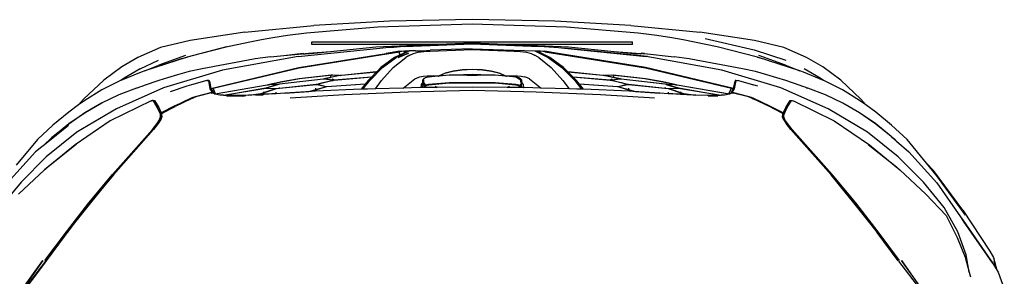
# Model space of a CAD drawing. Units: inches. Extents: x 1319 to 2030, y 219 to 1069.
# Tile 17 of 28: x 1433 to 1496, y 515 to 531. Entities that reach past the tile are written whole.
import ezdxf

# ---------------------------------------------------------------- set-up
doc = ezdxf.new("R2010")
doc.units = ezdxf.units.IN
doc.header["$MEASUREMENT"] = 0
doc.layers.get('0').update_dxf_attribs({"color": 12})
doc.layers.add('C-PRKG-VEHC', color=8, linetype='Continuous', lineweight=13)
doc.layers.add('Edges', color=250, linetype='Continuous')

# ---------------------------------------------------------------- blocks, each defined once
blk = doc.blocks.new('Nissan Qashqai pl')
at = {"layer": 'Edges'}
for p, q in [((7.6953, 12.7753), (7.7223, 12.7851)), ((7.5946, 12.718), (7.6608, 12.7617)), ((7.6113, 12.7186), (7.6759, 12.7633)), ((7.6799, 12.7658), (7.6125, 12.719)), ((7.6608, 12.7617), (7.6712, 12.7675)), ((7.6712, 12.7675), (7.6721, 12.7679)), ((7.6926, 12.7737), (7.6721, 12.7679)), ((7.6759, 12.7633), (7.6793, 12.7657)), ((7.6911, 12.7728), (7.6774, 12.7688)), ((7.6793, 12.7657), (7.6802, 12.766)), ((7.6799, 12.7658), (7.6802, 12.766)), ((7.6802, 12.766), (7.6809, 12.7664)), ((7.6809, 12.7664), (7.6911, 12.7728)), ((7.6911, 12.7728), (7.6926, 12.7737)), ((7.6926, 12.7737), (7.6953, 12.7753)), ((7.6949, 12.7283), (7.701, 12.73)), ((7.701, 12.73), (7.7024, 12.7301)), ((7.5946, 12.718), (7.5304, 12.6704)), ((7.6024, 12.7221), (7.5387, 12.6759)), ((7.5501, 12.6757), (7.6051, 12.7139)), ((7.6051, 12.7139), (7.6113, 12.7186)), ((7.6051, 12.7139), (7.6111, 12.7181)), ((7.6118, 12.7186), (7.6111, 12.7181)), ((7.6125, 12.719), (7.6118, 12.7186)), ((7.667, 12.723), (7.6295, 12.7097)), ((7.6386, 12.7089), (7.6708, 12.7217)), ((7.6949, 12.7283), (7.667, 12.723)), ((7.6708, 12.7217), (7.6949, 12.7283)), ((7.6295, 12.7097), (7.59, 12.6877)), ((7.6032, 12.6908), (7.6386, 12.7089)), ((7.59, 12.6877), (7.5492, 12.654)), ((7.5687, 12.6579), (7.6032, 12.6908)), ((7.5501, 12.6757), (7.5001, 12.6302)), ((7.5387, 12.6759), (7.5184, 12.6591)), ((7.5184, 12.6591), (7.5304, 12.6704)), ((7.5184, 12.6591), (7.4801, 12.6274)), ((7.5289, 12.6158), (7.5687, 12.6579)), ((7.5492, 12.654), (7.531, 12.6359)), ((7.7261, 12.6543), (7.6762, 12.6186)), ((7.6762, 12.6186), (7.7233, 12.6514)), ((7.531, 12.6359), (7.5081, 12.6131)), ((7.531, 12.6359), (7.5301, 12.6353)), ((7.6771, 12.6135), (7.7215, 12.6473)), ((7.4801, 12.6274), (7.4565, 12.6023)), ((7.4827, 12.6103), (7.5001, 12.6302)), ((7.4565, 12.6023), (7.4354, 12.5766)), ((7.4542, 12.5765), (7.4744, 12.6015)), ((7.475, 12.6016), (7.4549, 12.5767)), ((7.5081, 12.6131), (7.4679, 12.5634)), ((7.4744, 12.6015), (7.4804, 12.6079)), ((7.4762, 12.6028), (7.475, 12.6016)), ((7.4752, 12.6016), (7.4762, 12.6028)), ((7.4762, 12.6028), (7.478, 12.6049)), ((7.4804, 12.6079), (7.478, 12.6049)), ((7.478, 12.6049), (7.479, 12.6061)), ((7.479, 12.6061), (7.4815, 12.6089)), ((7.479, 12.6061), (7.4801, 12.6074)), ((7.4801, 12.6074), (7.4804, 12.6079)), ((7.4804, 12.6079), (7.4807, 12.6082)), ((7.4804, 12.6079), (7.4804, 12.6079)), ((7.4807, 12.6082), (7.4821, 12.6097)), ((7.4815, 12.6089), (7.4821, 12.6097)), ((7.4821, 12.6097), (7.4827, 12.6103)), ((7.4882, 12.5645), (7.5243, 12.6101)), ((7.4884, 12.5664), (7.5289, 12.6158)), ((7.5243, 12.6101), (7.5286, 12.6146)), ((7.676, 12.6152), (7.6296, 12.5803)), ((7.6769, 12.6129), (7.6306, 12.5791)), ((7.4354, 12.5766), (7.4239, 12.5604)), ((7.4363, 12.5502), (7.4542, 12.5765)), ((7.4549, 12.5767), (7.4369, 12.5504)), ((7.6296, 12.5803), (7.5827, 12.5441)), ((7.618, 12.5691), (7.5829, 12.5411)), ((7.618, 12.5691), (7.584, 12.5429)), ((7.6301, 12.5787), (7.618, 12.5691)), ((7.6306, 12.5791), (7.6301, 12.5787)), ((7.4239, 12.5604), (7.4147, 12.5524)), ((7.4239, 12.5604), (7.4166, 12.5503)), ((7.4679, 12.5634), (7.4302, 12.4993)), ((7.4498, 12.5093), (7.4884, 12.5664)), ((7.4147, 12.5524), (7.3837, 12.5197)), ((7.4166, 12.5503), (7.3997, 12.5227)), ((7.4205, 12.5229), (7.4363, 12.5502)), ((7.4369, 12.5504), (7.4211, 12.5232)), ((7.5827, 12.5441), (7.5369, 12.5057)), ((7.584, 12.5429), (7.5568, 12.5201)), ((7.5829, 12.5411), (7.5568, 12.5201)), ((7.3997, 12.5227), (7.3845, 12.4925)), ((7.4071, 12.4948), (7.4205, 12.5229)), ((7.4211, 12.5232), (7.4078, 12.4951)), ((7.3837, 12.5197), (7.3624, 12.4907)), ((7.4172, 12.4431), (7.4498, 12.5093)), ((7.5369, 12.5057), (7.4635, 12.4408)), ((7.5568, 12.5201), (7.5371, 12.5042)), ((7.3624, 12.4907), (7.347, 12.4644)), ((7.3843, 12.492), (7.3707, 12.4592)), ((7.3843, 12.492), (7.3805, 12.4866)), ((7.3845, 12.4925), (7.3843, 12.492)), ((7.3962, 12.466), (7.4071, 12.4948)), ((7.4302, 12.4993), (7.3963, 12.4227)), ((7.4078, 12.4951), (7.3969, 12.4665)), ((7.4638, 12.439), (7.5371, 12.5042)), ((7.3805, 12.4866), (7.3655, 12.4604)), ((7.347, 12.4644), (7.3309, 12.4276)), ((7.3707, 12.4592), (7.3688, 12.4532)), ((7.3938, 12.4583), (7.3925, 12.4542)), ((7.3951, 12.462), (7.3938, 12.4583)), ((7.3965, 12.4655), (7.3951, 12.462)), ((7.3965, 12.4655), (7.3962, 12.466)), ((7.3969, 12.4665), (7.3965, 12.4655)), ((7.3968, 12.4649), (7.3967, 12.4651)), ((7.3688, 12.4532), (7.3467, 12.3846)), ((7.3596, 12.4302), (7.3688, 12.4532)), ((7.3925, 12.4542), (7.3845, 12.4306)), ((7.4169, 12.4412), (7.4172, 12.4431)), ((7.4169, 12.4406), (7.4172, 12.4423)), ((7.4169, 12.4406), (7.4169, 12.4412)), ((7.4172, 12.4423), (7.4174, 12.4429)), ((7.4175, 12.4429), (7.4174, 12.4429)), ((7.3309, 12.4276), (7.3193, 12.3797)), ((7.3345, 12.3793), (7.3514, 12.4308)), ((7.3596, 12.4302), (7.344, 12.3869)), ((7.3845, 12.4306), (7.3799, 12.4164)), ((7.4167, 12.4393), (7.4169, 12.4406)), ((7.4167, 12.4393), (7.4172, 12.4395)), ((7.417, 12.4377), (7.4167, 12.4393)), ((7.4169, 12.4398), (7.4169, 12.4406)), ((7.4282, 12.4328), (7.4169, 12.4398)), ((7.4172, 12.4395), (7.4169, 12.4398)), ((7.4283, 12.4307), (7.417, 12.4377)), ((7.4183, 12.4382), (7.4172, 12.4395)), ((7.4183, 12.4382), (7.4296, 12.4312)), ((7.4255, 12.4044), (7.4367, 12.4268)), ((7.4387, 12.428), (7.4282, 12.4328)), ((7.4359, 12.4272), (7.4283, 12.4307)), ((7.4383, 12.4272), (7.4296, 12.4312)), ((7.4367, 12.4268), (7.4359, 12.4272)), ((7.4378, 12.4261), (7.4365, 12.4235)), ((7.4367, 12.4268), (7.4383, 12.4272)), ((7.4379, 12.4263), (7.4378, 12.4261)), ((7.4379, 12.4263), (7.4383, 12.4272)), ((7.4379, 12.4263), (7.4389, 12.4269)), ((7.4384, 12.426), (7.4379, 12.4263)), ((7.4384, 12.426), (7.438, 12.4251)), ((7.4383, 12.4272), (7.4389, 12.4269)), ((7.4389, 12.4269), (7.4384, 12.426)), ((7.4387, 12.4259), (7.4384, 12.426)), ((7.4431, 12.4276), (7.4387, 12.428)), ((7.443, 12.4254), (7.4387, 12.4259)), ((7.44, 12.4264), (7.4389, 12.4269)), ((7.44, 12.4264), (7.4442, 12.4258)), ((7.4477, 12.427), (7.443, 12.4254)), ((7.4479, 12.4293), (7.4431, 12.4276)), ((7.4442, 12.4258), (7.4477, 12.427)), ((7.4477, 12.427), (7.4541, 12.4313)), ((7.4541, 12.4333), (7.4479, 12.4293)), ((7.4635, 12.4408), (7.4541, 12.4333)), ((7.4638, 12.439), (7.4541, 12.4313)), ((7.3963, 12.4227), (7.3676, 12.3269)), ((7.3799, 12.4164), (7.375, 12.4)), ((7.4365, 12.4235), (7.4267, 12.4041)), ((7.4365, 12.4235), (7.4365, 12.4235)), ((7.375, 12.4), (7.3699, 12.3813)), ((7.4131, 12.3783), (7.4255, 12.4044)), ((7.4267, 12.4041), (7.4139, 12.3778)), ((7.3193, 12.3797), (7.3059, 12.291)), ((7.3161, 12.3001), (7.3345, 12.3793)), ((7.3467, 12.3846), (7.33, 12.3192)), ((7.3467, 12.3846), (7.3489, 12.3925)), ((7.3699, 12.3813), (7.3653, 12.3604)), ((7.3913, 12.3774), (7.3844, 12.3526)), ((7.3913, 12.3774), (7.3914, 12.3775)), ((7.3925, 12.3813), (7.3914, 12.3775)), ((7.3937, 12.3851), (7.3925, 12.3813)), ((7.4115, 12.3746), (7.4131, 12.3783)), ((7.4139, 12.3778), (7.4122, 12.3742)), ((7.4133, 12.3759), (7.4142, 12.3776)), ((7.4033, 12.3435), (7.4101, 12.3708)), ((7.4108, 12.3703), (7.4042, 12.3435)), ((7.4101, 12.3708), (7.4115, 12.3746)), ((7.4122, 12.3742), (7.4108, 12.3703)), ((7.3653, 12.3604), (7.3497, 12.2767)), ((7.3971, 12.3461), (7.3635, 12.2033)), ((7.3841, 12.3485), (7.3844, 12.3526)), ((7.3846, 12.3495), (7.3841, 12.3485)), ((7.3841, 12.3485), (7.3853, 12.3483)), ((7.3846, 12.3495), (7.3976, 12.347)), ((7.3971, 12.3461), (7.3853, 12.3483)), ((7.3983, 12.3458), (7.3971, 12.3461)), ((7.3976, 12.347), (7.4026, 12.3439)), ((7.4012, 12.3441), (7.3983, 12.3458)), ((7.4045, 12.3434), (7.405, 12.3456)), ((7.364, 12.2029), (7.3968, 12.3424)), ((7.3916, 12.2547), (7.4062, 12.3389)), ((7.4065, 12.3392), (7.3917, 12.2547)), ((7.3968, 12.3424), (7.398, 12.3449)), ((7.4046, 12.3389), (7.3968, 12.3424)), ((7.398, 12.3449), (7.3999, 12.344)), ((7.398, 12.3449), (7.4012, 12.3441)), ((7.3999, 12.344), (7.4051, 12.3415)), ((7.3999, 12.344), (7.4048, 12.3417)), ((7.4033, 12.3427), (7.4012, 12.3441)), ((7.4012, 12.3441), (7.4015, 12.344)), ((7.4015, 12.344), (7.4028, 12.3437)), ((7.4026, 12.3439), (7.4033, 12.3435)), ((7.4033, 12.3435), (7.4042, 12.3422)), ((7.4042, 12.3422), (7.4033, 12.3427)), ((7.4042, 12.3435), (7.404, 12.3429)), ((7.404, 12.3429), (7.4043, 12.3428)), ((7.404, 12.3429), (7.4043, 12.3425)), ((7.4041, 12.3435), (7.4042, 12.3435)), ((7.4042, 12.3435), (7.4045, 12.3434)), ((7.4042, 12.3422), (7.4043, 12.3425)), ((7.4044, 12.3422), (7.4042, 12.3422)), ((7.4043, 12.3428), (7.4045, 12.3434)), ((7.4043, 12.3428), (7.4046, 12.3425)), ((7.4043, 12.3425), (7.4043, 12.3428)), ((7.4043, 12.3425), (7.4044, 12.3422)), ((7.4044, 12.3422), (7.4046, 12.3419)), ((7.4046, 12.3422), (7.4044, 12.3422)), ((7.4045, 12.3434), (7.4048, 12.3433)), ((7.4046, 12.3425), (7.4047, 12.3424)), ((7.4047, 12.3424), (7.4046, 12.3422)), ((7.4046, 12.3422), (7.4046, 12.3419)), ((7.4048, 12.3422), (7.4046, 12.3422)), ((7.4046, 12.3419), (7.405, 12.3419)), ((7.4048, 12.3417), (7.4046, 12.3419)), ((7.4046, 12.3389), (7.4062, 12.3389)), ((7.4047, 12.3424), (7.4048, 12.3422)), ((7.4048, 12.3422), (7.405, 12.3419)), ((7.4048, 12.3417), (7.4052, 12.3416)), ((7.4051, 12.3415), (7.4048, 12.3417)), ((7.405, 12.3419), (7.4052, 12.3416)), ((7.4051, 12.3415), (7.4052, 12.3415)), ((7.4052, 12.3416), (7.4052, 12.3415)), ((7.4052, 12.3415), (7.4063, 12.3395)), ((7.4062, 12.3389), (7.4063, 12.3395)), ((7.4063, 12.3395), (7.4065, 12.3392)), ((7.4065, 12.3392), (7.4066, 12.3389)), ((7.4066, 12.3389), (7.408, 12.3313)), ((7.408, 12.3313), (7.4083, 12.3258)), ((7.33, 12.3192), (7.3261, 12.3009)), ((7.3676, 12.3269), (7.3455, 12.2042)), ((7.3971, 12.2599), (7.4083, 12.3258)), ((7.4084, 12.3244), (7.3975, 12.2599)), ((7.4083, 12.3258), (7.4084, 12.3244)), ((7.4084, 12.3244), (7.4087, 12.3195)), ((7.4087, 12.3195), (7.4087, 12.3037)), ((7.4092, 12.3184), (7.4091, 12.3206)), ((7.4092, 12.305), (7.4092, 12.3184)), ((7.3261, 12.3009), (7.3223, 12.2825)), ((7.4087, 12.3037), (7.4081, 12.2848)), ((7.2951, 12.1791), (7.3059, 12.291)), ((7.3223, 12.2825), (7.3186, 12.2641)), ((7.4054, 12.2651), (7.4081, 12.2848)), ((7.4081, 12.2838), (7.4079, 12.2798)), ((7.4081, 12.2848), (7.4081, 12.2838)), ((7.3494, 12.2741), (7.3457, 12.2495)), ((7.3498, 12.2768), (7.3494, 12.2741)), ((7.3497, 12.2767), (7.3494, 12.2741)), ((7.4079, 12.2798), (7.4059, 12.2651)), ((7.4079, 12.2798), (7.4069, 12.2598)), ((7.3186, 12.2641), (7.3149, 12.2457)), ((7.3909, 12.2508), (7.3864, 12.231)), ((7.3869, 12.2347), (7.3912, 12.2527)), ((7.3901, 12.2368), (7.391, 12.2507)), ((7.3914, 12.2527), (7.3906, 12.2386)), ((7.3908, 12.2366), (7.3965, 12.256)), ((7.3911, 12.2518), (7.3909, 12.2508)), ((7.391, 12.2387), (7.3967, 12.2579)), ((7.391, 12.2507), (7.3911, 12.2518)), ((7.3912, 12.2517), (7.3911, 12.2518)), ((7.3912, 12.2527), (7.3916, 12.2547)), ((7.3917, 12.2547), (7.3914, 12.2527)), ((7.3969, 12.257), (7.3965, 12.256)), ((7.3967, 12.2579), (7.3971, 12.2599)), ((7.3968, 12.2559), (7.3969, 12.257)), ((7.3972, 12.2421), (7.3968, 12.2559)), ((7.3975, 12.2599), (7.3973, 12.258)), ((7.3973, 12.258), (7.3977, 12.2439)), ((7.4048, 12.2612), (7.3982, 12.2419)), ((7.3983, 12.244), (7.4038, 12.2599)), ((7.4028, 12.2599), (7.4038, 12.2599)), ((7.4038, 12.2599), (7.4049, 12.2631)), ((7.4053, 12.2622), (7.4048, 12.2612)), ((7.4049, 12.2631), (7.4054, 12.2651)), ((7.4053, 12.2612), (7.4053, 12.2622)), ((7.4061, 12.2473), (7.4053, 12.2612)), ((7.4059, 12.2618), (7.4056, 12.2621)), ((7.4059, 12.2651), (7.4058, 12.2632)), ((7.4058, 12.2632), (7.4059, 12.2618)), ((7.4059, 12.2618), (7.4064, 12.2523)), ((7.4064, 12.2523), (7.4061, 12.2473)), ((7.4069, 12.2598), (7.4064, 12.2523)), ((7.3149, 12.2457), (7.3113, 12.2217)), ((7.3407, 12.2016), (7.3457, 12.2495)), ((7.3813, 12.2021), (7.3869, 12.2347)), ((7.3815, 12.1638), (7.3899, 12.2348)), ((7.3903, 12.2347), (7.382, 12.1639)), ((7.3899, 12.2348), (7.3901, 12.2368)), ((7.3908, 12.2366), (7.3903, 12.2347)), ((7.3905, 12.1754), (7.3966, 12.2347)), ((7.3906, 12.2386), (7.3907, 12.2376)), ((7.3907, 12.2376), (7.391, 12.2387)), ((7.3977, 12.24), (7.3911, 12.1755)), ((7.3957, 12.2348), (7.3966, 12.2348)), ((7.3957, 12.2347), (7.3966, 12.2347)), ((7.3966, 12.2348), (7.3972, 12.24)), ((7.3966, 12.2347), (7.3966, 12.2348)), ((7.3972, 12.24), (7.3972, 12.2421)), ((7.3977, 12.2439), (7.398, 12.2429)), ((7.3982, 12.2419), (7.3977, 12.24)), ((7.398, 12.2429), (7.3983, 12.244)), ((7.4032, 12.24), (7.4057, 12.24)), ((7.4057, 12.24), (7.4048, 12.2262)), ((7.4061, 12.2472), (7.4057, 12.24)), ((7.4061, 12.2472), (7.4061, 12.2473)), ((7.3113, 12.2217), (7.3078, 12.191)), ((7.3864, 12.231), (7.3815, 12.2029)), ((7.4022, 12.187), (7.4048, 12.2262)), ((7.4048, 12.2262), (7.4023, 12.1836)), ((7.4072, 12.1299), (7.4124, 12.2176)), ((7.3455, 12.2062), (7.3317, 12.0717)), ((7.3317, 12.0717), (7.3455, 12.2042)), ((7.3635, 12.2033), (7.3405, 12.0616)), ((7.3426, 12.0707), (7.364, 12.2029)), ((7.375, 12.1484), (7.3813, 12.2021)), ((7.3815, 12.2029), (7.3756, 12.1509)), ((7.3078, 12.191), (7.298, 12.075)), ((7.3407, 12.1879), (7.3378, 12.1521)), ((7.3407, 12.2016), (7.34, 12.1962)), ((7.34, 12.1962), (7.3401, 12.1962)), ((7.3401, 12.1962), (7.341, 12.1962)), ((7.3403, 12.1981), (7.3407, 12.2016)), ((7.3413, 12.1933), (7.3407, 12.1879)), ((7.341, 12.1962), (7.3414, 12.1962)), ((7.341, 12.1962), (7.341, 12.1962)), ((7.3414, 12.1962), (7.341, 12.1962)), ((7.341, 12.1962), (7.3413, 12.1933)), ((7.3413, 12.1931), (7.341, 12.1848)), ((7.3415, 12.1954), (7.3413, 12.1933)), ((7.3413, 12.1933), (7.3413, 12.1931)), ((7.4017, 12.185), (7.4022, 12.187)), ((7.2951, 12.1791), (7.2884, 12.0562)), ((7.3261, 12.1821), (7.3216, 12.1821)), ((7.3216, 11.6621), (7.3216, 12.1821)), ((7.3261, 12.1821), (7.3261, 11.9779)), ((7.34, 12.1731), (7.3378, 12.1521)), ((7.341, 12.1848), (7.34, 12.1731)), ((7.3903, 12.1716), (7.3844, 12.1479)), ((7.3877, 12.1639), (7.3901, 12.1734)), ((7.3901, 12.1734), (7.3905, 12.1754)), ((7.3907, 12.1727), (7.3903, 12.1716)), ((7.3909, 12.1716), (7.3907, 12.1727)), ((7.3939, 12.1596), (7.3909, 12.1716)), ((7.3911, 12.1755), (7.3913, 12.1737)), ((7.3913, 12.1737), (7.3943, 12.1614)), ((7.3949, 12.1616), (7.399, 12.1756)), ((7.4021, 12.1833), (7.3951, 12.1606)), ((7.3967, 12.1756), (7.399, 12.1756)), ((7.4018, 12.1764), (7.3986, 12.1025)), ((7.399, 12.1756), (7.4017, 12.185)), ((7.4023, 12.1836), (7.4018, 12.1764)), ((7.4023, 12.1836), (7.4021, 12.1833)), ((7.3813, 12.1599), (7.3763, 12.1361)), ((7.3792, 12.1518), (7.3812, 12.1619)), ((7.3812, 12.1619), (7.3815, 12.1638)), ((7.3815, 12.161), (7.3813, 12.1599)), ((7.3817, 12.16), (7.3815, 12.161)), ((7.3832, 12.1493), (7.3817, 12.16)), ((7.382, 12.1639), (7.382, 12.1619)), ((7.382, 12.1619), (7.3838, 12.1497)), ((7.3843, 12.1498), (7.3877, 12.1639)), ((7.3877, 12.1639), (7.3874, 12.1639)), ((7.3896, 12.0954), (7.3941, 12.1576)), ((7.3945, 12.1577), (7.3903, 12.0959)), ((7.3941, 12.1576), (7.3939, 12.1596)), ((7.3943, 12.1614), (7.3947, 12.1605)), ((7.3951, 12.1606), (7.3945, 12.1577)), ((7.3947, 12.1605), (7.3949, 12.1616)), ((7.3378, 12.1521), (7.3302, 12.0785)), ((7.376, 12.136), (7.375, 12.1484)), ((7.3756, 12.1509), (7.3792, 12.1518)), ((7.3756, 12.1509), (7.3762, 12.138)), ((7.3762, 12.137), (7.3764, 12.138)), ((7.3762, 12.138), (7.3762, 12.137)), ((7.3764, 12.138), (7.3792, 12.1518)), ((7.3783, 12.0852), (7.3836, 12.1459)), ((7.384, 12.1459), (7.3788, 12.0857)), ((7.3832, 12.1493), (7.3824, 12.1487)), ((7.3824, 12.1487), (7.3832, 12.1492)), ((7.3836, 12.1459), (7.3824, 12.1487)), ((7.3824, 12.1487), (7.3835, 12.1468)), ((7.3838, 12.1497), (7.3832, 12.1493)), ((7.3832, 12.1492), (7.3837, 12.1495)), ((7.3832, 12.1492), (7.3832, 12.1493)), ((7.3836, 12.1459), (7.3835, 12.1468)), ((7.3835, 12.1468), (7.384, 12.1459)), ((7.3837, 12.1495), (7.3843, 12.1498)), ((7.3837, 12.1495), (7.3838, 12.1497)), ((7.384, 12.1459), (7.3842, 12.1495)), ((7.3844, 12.1479), (7.384, 12.1459)), ((7.3842, 12.1495), (7.3843, 12.1498)), ((7.3843, 12.1495), (7.3842, 12.1495)), ((7.3701, 12.0771), (7.3759, 12.1341)), ((7.3761, 12.1341), (7.3704, 12.0773)), ((7.3759, 12.1341), (7.376, 12.136)), ((7.3763, 12.1361), (7.3761, 12.1341)), ((7.3764, 12.1371), (7.3762, 12.137)), ((7.4025, 12.026), (7.4072, 12.1299)), ((7.3841, 12.091), (7.3788, 12.0857)), ((7.3896, 12.0954), (7.3841, 12.091)), ((7.3845, 12.0883), (7.3985, 12.0993)), ((7.3903, 12.0959), (7.3896, 12.0954)), ((7.3986, 12.1025), (7.3903, 12.0959)), ((7.3982, 12.092), (7.3978, 12.0791)), ((7.3985, 12.0993), (7.3982, 12.092)), ((7.3986, 12.1025), (7.3985, 12.0993)), ((7.298, 12.075), (7.2928, 11.9221)), ((7.3302, 12.0785), (7.3261, 11.9779)), ((7.3701, 12.0771), (7.3631, 12.0701)), ((7.3633, 12.0674), (7.3845, 12.0883)), ((7.3704, 12.0773), (7.3701, 12.0771)), ((7.3783, 12.0852), (7.3704, 12.0773)), ((7.3788, 12.0857), (7.3783, 12.0852)), ((7.3842, 12.0693), (7.3978, 12.0791)), ((7.3978, 12.0791), (7.3966, 12.0338)), ((7.3294, 12.0385), (7.3309, 12.0619)), ((7.3309, 12.0619), (7.3317, 12.0717)), ((7.3405, 12.0616), (7.3369, 12.0394)), ((7.3377, 12.0398), (7.341, 12.0605)), ((7.341, 12.0605), (7.3426, 12.0707)), ((7.3631, 12.0701), (7.3469, 12.0481)), ((7.3471, 12.0454), (7.3633, 12.0674)), ((7.363, 12.0501), (7.3842, 12.0693)), ((7.2884, 12.0562), (7.2857, 11.9221)), ((7.3365, 12.0237), (7.3471, 12.0454)), ((7.3469, 12.0481), (7.3402, 12.0337)), ((7.3468, 12.0299), (7.363, 12.0501)), ((7.3251, 11.9221), (7.3291, 12.0316)), ((7.3294, 12.0385), (7.3291, 12.0316)), ((7.3362, 12.0248), (7.3365, 12.0321)), ((7.3365, 12.0321), (7.3369, 12.0394)), ((7.3377, 12.0398), (7.3369, 12.0328)), ((7.3369, 12.0287), (7.3369, 12.0328)), ((7.338, 12.0291), (7.3369, 12.0287)), ((7.3374, 12.0276), (7.3369, 12.0287)), ((7.338, 12.0291), (7.3374, 12.0276)), ((7.3402, 12.0337), (7.338, 12.0291)), ((7.3387, 12.0332), (7.3402, 12.0337)), ((7.3468, 12.0299), (7.3432, 12.0231)), ((7.3818, 12.0151), (7.3966, 12.0338)), ((7.3966, 12.0338), (7.3959, 12.0071)), ((7.4002, 11.9221), (7.4025, 12.026)), ((7.3329, 11.9221), (7.3365, 12.0237)), ((7.3362, 12.0248), (7.3366, 12.0246)), ((7.3365, 12.0237), (7.3362, 12.0248)), ((7.3373, 12.0004), (7.3386, 12.01)), ((7.3386, 12.01), (7.3407, 12.0176)), ((7.3407, 12.0176), (7.3432, 12.0231)), ((7.3801, 12.0115), (7.3786, 12.007)), ((7.3818, 12.0151), (7.3801, 12.0115)), ((7.3367, 11.99), (7.3373, 12.0004)), ((7.3765, 11.989), (7.3768, 11.9954)), ((7.3768, 11.9954), (7.3775, 12.0015)), ((7.3775, 12.0015), (7.3786, 12.007)), ((7.3798, 11.9983), (7.3787, 11.9928)), ((7.3787, 11.9928), (7.38, 11.9953)), ((7.3808, 11.9993), (7.3798, 11.9983)), ((7.3807, 11.9991), (7.3798, 11.9983)), ((7.38, 11.9953), (7.383, 12.0011)), ((7.3807, 11.9991), (7.3808, 11.9993)), ((7.381, 11.9993), (7.3807, 11.9991)), ((7.3808, 11.9993), (7.384, 12.0021)), ((7.381, 11.9993), (7.3808, 11.9993)), ((7.383, 12.0011), (7.381, 11.9993)), ((7.3866, 12.0011), (7.383, 12.0011)), ((7.384, 12.0021), (7.387, 12.0021)), ((7.3868, 12.002), (7.3866, 12.0011)), ((7.3875, 12.0011), (7.3866, 12.0011)), ((7.387, 12.0021), (7.3868, 12.002)), ((7.3909, 12.0051), (7.387, 12.0021)), ((7.387, 12.0021), (7.3885, 12.0021)), ((7.3885, 12.0021), (7.3925, 11.9993)), ((7.3955, 12.0021), (7.3885, 12.0021)), ((7.3904, 11.9928), (7.3916, 11.9983)), ((7.3956, 12.0051), (7.3909, 12.0051)), ((7.3929, 11.9981), (7.3917, 11.9926)), ((7.3925, 11.9993), (7.3958, 11.9993)), ((7.3925, 11.9993), (7.3929, 11.9981)), ((7.3958, 11.9981), (7.3929, 11.9981)), ((7.3955, 12.0021), (7.3958, 12.0018)), ((7.3959, 12.0049), (7.3956, 12.0051)), ((7.3959, 12.0051), (7.3956, 12.0051)), ((7.3958, 11.9981), (7.3956, 11.9801)), ((7.3959, 12.0049), (7.3958, 12.0018)), ((7.3958, 12.0018), (7.3958, 11.9993)), ((7.3958, 11.9993), (7.3958, 11.9981)), ((7.3959, 12.0071), (7.3959, 12.0051)), ((7.3959, 12.0051), (7.3959, 12.0049)), ((7.3343, 11.9221), (7.3367, 11.99)), ((7.3761, 11.9751), (7.3765, 11.989)), ((7.3787, 11.9928), (7.3774, 11.9778)), ((7.3876, 11.9595), (7.3904, 11.9928)), ((7.3917, 11.9926), (7.3889, 11.9594)), ((7.3938, 11.9823), (7.3956, 11.9801)), ((7.3956, 11.9788), (7.3938, 11.981)), ((7.3956, 11.9788), (7.3951, 11.9221)), ((7.3956, 11.9801), (7.3956, 11.9788)), ((7.3261, 11.9764), (7.3238, 11.9221)), ((7.3261, 11.9764), (7.3261, 11.9779)), ((7.369, 11.9536), (7.3724, 11.9667)), ((7.3727, 11.9658), (7.3693, 11.953)), ((7.3724, 11.9667), (7.3761, 11.9751)), ((7.3771, 11.9757), (7.3727, 11.9658)), ((7.3773, 11.9759), (7.3759, 11.9595)), ((7.3761, 11.9751), (7.3769, 11.9767)), ((7.3769, 11.9767), (7.3771, 11.977)), ((7.3774, 11.9778), (7.3771, 11.9771)), ((7.3771, 11.9771), (7.3774, 11.9774)), ((7.3771, 11.9771), (7.3771, 11.977)), ((7.3773, 11.9759), (7.3771, 11.9757)), ((7.3774, 11.9774), (7.3773, 11.9759)), ((7.3774, 11.9774), (7.3774, 11.9778)), ((7.3668, 11.9384), (7.369, 11.9536)), ((7.3693, 11.953), (7.3672, 11.9381)), ((7.3759, 11.9595), (7.3759, 11.9417)), ((7.3876, 11.8847), (7.3876, 11.9595)), ((7.3889, 11.9594), (7.3889, 11.8848)), ((7.3661, 11.9221), (7.3668, 11.9384)), ((7.3672, 11.9381), (7.3665, 11.9221)), ((7.3751, 11.9363), (7.3745, 11.9221)), ((7.3759, 11.9417), (7.3751, 11.9363)), ((7.3755, 11.9221), (7.3759, 11.9303)), ((7.3759, 11.9417), (7.3759, 11.9303)), ((7.3759, 11.9303), (7.3759, 11.9139)), ((7.2857, 11.9221), (7.2884, 11.7879)), ((7.2928, 11.9221), (7.298, 11.7692)), ((7.3238, 11.9221), (7.3261, 11.8662)), ((7.3291, 11.8126), (7.3251, 11.9221)), ((7.3329, 11.9221), (7.3354, 11.8539)), ((7.3367, 11.8541), (7.3343, 11.9221)), ((7.3668, 11.9057), (7.3661, 11.9221)), ((7.3665, 11.9221), (7.3672, 11.9061)), ((7.3745, 11.9221), (7.3751, 11.9078)), ((7.3759, 11.9139), (7.3755, 11.9221)), ((7.3951, 11.9221), (7.3956, 11.8653)), ((7.4025, 11.8181), (7.4002, 11.9221)), ((7.369, 11.8905), (7.3668, 11.9057)), ((7.3672, 11.9061), (7.3693, 11.8911)), ((7.3751, 11.9078), (7.3759, 11.9025)), ((7.3759, 11.9139), (7.3759, 11.9025)), ((7.3759, 11.9025), (7.3759, 11.8847)), ((7.3724, 11.8775), (7.369, 11.8905)), ((7.3693, 11.8911), (7.3727, 11.8783)), ((7.3759, 11.8847), (7.3773, 11.8682)), ((7.3904, 11.8513), (7.3876, 11.8847)), ((7.3889, 11.8848), (7.3917, 11.8516)), ((7.3261, 11.8662), (7.3302, 11.7656)), ((7.3261, 11.8662), (7.3261, 11.6621)), ((7.3761, 11.8691), (7.3724, 11.8775)), ((7.3727, 11.8783), (7.3771, 11.8685)), ((7.3765, 11.8551), (7.3761, 11.8691)), ((7.3769, 11.8674), (7.3761, 11.8691)), ((7.3771, 11.8671), (7.3769, 11.8674)), ((7.3771, 11.8685), (7.3773, 11.8682)), ((7.3771, 11.8671), (7.3771, 11.8671)), ((7.3771, 11.8671), (7.3774, 11.8664)), ((7.3774, 11.8668), (7.3771, 11.8671)), ((7.3773, 11.8682), (7.3774, 11.8668)), ((7.3774, 11.8668), (7.3774, 11.8664)), ((7.3774, 11.8664), (7.3787, 11.8513)), ((7.3361, 11.8416), (7.3354, 11.8539)), ((7.3373, 11.8438), (7.3367, 11.8541)), ((7.3768, 11.8488), (7.3765, 11.8551)), ((7.3787, 11.8513), (7.3798, 11.8459)), ((7.3916, 11.8459), (7.3904, 11.8513)), ((7.3917, 11.8516), (7.3929, 11.8461)), ((7.3938, 11.8632), (7.3956, 11.8653)), ((7.3956, 11.864), (7.3938, 11.8619)), ((7.3956, 11.8653), (7.3956, 11.864)), ((7.3956, 11.864), (7.3958, 11.8461)), ((7.3362, 11.8301), (7.3361, 11.8416)), ((7.3386, 11.8342), (7.3373, 11.8438)), ((7.3775, 11.8427), (7.3768, 11.8488)), ((7.3786, 11.8372), (7.3775, 11.8427)), ((7.3801, 11.8327), (7.3786, 11.8372)), ((7.3798, 11.8459), (7.3808, 11.8448)), ((7.3808, 11.8448), (7.3807, 11.8451)), ((7.3808, 11.8448), (7.381, 11.8448)), ((7.384, 11.8421), (7.3808, 11.8448)), ((7.383, 11.8431), (7.3875, 11.8431)), ((7.387, 11.8421), (7.384, 11.8421)), ((7.387, 11.8421), (7.3909, 11.8391)), ((7.3885, 11.8421), (7.387, 11.8421)), ((7.3875, 11.8431), (7.3916, 11.8459)), ((7.3925, 11.8448), (7.3885, 11.8421)), ((7.3955, 11.8421), (7.3885, 11.8421)), ((7.3909, 11.8391), (7.3956, 11.8391)), ((7.3929, 11.8461), (7.3925, 11.8448)), ((7.3958, 11.8448), (7.3925, 11.8448)), ((7.3929, 11.8461), (7.3958, 11.8461)), ((7.3958, 11.8423), (7.3955, 11.8421)), ((7.3956, 11.8391), (7.3959, 11.8392)), ((7.3956, 11.8391), (7.3959, 11.8391)), ((7.3958, 11.8461), (7.3958, 11.8448)), ((7.3958, 11.8448), (7.3958, 11.8423)), ((7.3958, 11.8423), (7.3959, 11.8392)), ((7.3959, 11.8392), (7.3959, 11.8391)), ((7.3959, 11.8391), (7.3959, 11.8371)), ((7.3959, 11.8371), (7.3966, 11.8103)), ((7.3362, 11.8301), (7.3365, 11.8204)), ((7.3362, 11.8194), (7.3365, 11.8204)), ((7.3367, 11.8196), (7.3362, 11.8194)), ((7.3365, 11.812), (7.3362, 11.8194)), ((7.3365, 11.8204), (7.3471, 11.7987)), ((7.3407, 11.8266), (7.3386, 11.8342)), ((7.3401, 11.8186), (7.3431, 11.8112)), ((7.347, 11.8021), (7.3401, 11.8186)), ((7.3432, 11.821), (7.3407, 11.8266)), ((7.3432, 11.821), (7.3468, 11.8142)), ((7.3818, 11.8291), (7.3801, 11.8327)), ((7.3966, 11.8103), (7.3818, 11.8291)), ((7.3291, 11.8126), (7.3294, 11.8057)), ((7.3301, 11.7949), (7.3294, 11.8057)), ((7.3369, 11.8047), (7.3365, 11.812)), ((7.3369, 11.8155), (7.3374, 11.8165)), ((7.3369, 11.8113), (7.3369, 11.8155)), ((7.3369, 11.8155), (7.338, 11.8151)), ((7.3369, 11.8113), (7.3377, 11.8044)), ((7.3369, 11.8047), (7.3405, 11.7825)), ((7.3374, 11.8165), (7.338, 11.8151)), ((7.3377, 11.8042), (7.3377, 11.8044)), ((7.341, 11.7837), (7.3377, 11.8042)), ((7.338, 11.8151), (7.343, 11.8045)), ((7.343, 11.8045), (7.3396, 11.8043)), ((7.3396, 11.8043), (7.3431, 11.8042)), ((7.343, 11.8045), (7.3431, 11.8042)), ((7.3431, 11.8112), (7.347, 11.8021)), ((7.3431, 11.8042), (7.3469, 11.7961)), ((7.363, 11.794), (7.3468, 11.8142)), ((7.3966, 11.8103), (7.3978, 11.7651)), ((7.4072, 11.7142), (7.4025, 11.8181)), ((7.2884, 11.7879), (7.2951, 11.6651)), ((7.3295, 11.8012), (7.3309, 11.7822)), ((7.3295, 11.8012), (7.3301, 11.7949)), ((7.3309, 11.7822), (7.3301, 11.7949)), ((7.3469, 11.7961), (7.3631, 11.774)), ((7.3633, 11.7767), (7.3471, 11.7987)), ((7.3842, 11.7749), (7.363, 11.794)), ((7.3317, 11.7724), (7.3309, 11.7822)), ((7.3455, 11.64), (7.3317, 11.7724)), ((7.3635, 11.6409), (7.3405, 11.7825)), ((7.3426, 11.7735), (7.341, 11.7837)), ((7.364, 11.6413), (7.3426, 11.7735)), ((7.3631, 11.774), (7.3701, 11.7671)), ((7.3845, 11.7558), (7.3633, 11.7767)), ((7.3978, 11.7651), (7.3842, 11.7749)), ((7.298, 11.7692), (7.3078, 11.6532)), ((7.3302, 11.7656), (7.3378, 11.6921)), ((7.3759, 11.7101), (7.3701, 11.7671)), ((7.3701, 11.7671), (7.3704, 11.7668)), ((7.3704, 11.7668), (7.3761, 11.71)), ((7.3704, 11.7668), (7.3783, 11.759)), ((7.3836, 11.6983), (7.3783, 11.759)), ((7.3783, 11.759), (7.3788, 11.7585)), ((7.3788, 11.7585), (7.384, 11.6982)), ((7.3788, 11.7585), (7.3841, 11.7532)), ((7.3985, 11.7448), (7.3845, 11.7558)), ((7.3978, 11.7651), (7.3982, 11.7521)), ((7.3841, 11.7532), (7.3896, 11.7488)), ((7.3941, 11.6865), (7.3896, 11.7488)), ((7.3896, 11.7488), (7.3903, 11.7483)), ((7.3903, 11.7483), (7.3945, 11.6865)), ((7.3903, 11.7483), (7.3986, 11.7417)), ((7.3982, 11.7521), (7.3985, 11.7448)), ((7.3985, 11.7448), (7.3986, 11.7417)), ((7.3986, 11.7417), (7.4018, 11.6678)), ((7.375, 11.6957), (7.376, 11.7081)), ((7.376, 11.7081), (7.3759, 11.7101)), ((7.3761, 11.71), (7.3763, 11.7081)), ((7.3763, 11.7081), (7.3813, 11.6842)), ((7.4124, 11.6265), (7.4072, 11.7142)), ((7.3378, 11.6921), (7.3407, 11.6563)), ((7.3378, 11.6921), (7.34, 11.671)), ((7.3813, 11.642), (7.375, 11.6957)), ((7.3757, 11.6959), (7.3756, 11.6933)), ((7.3792, 11.6924), (7.3756, 11.6933)), ((7.3756, 11.6933), (7.3815, 11.6413)), ((7.3762, 11.7062), (7.3757, 11.6959)), ((7.3757, 11.6959), (7.3757, 11.6959)), ((7.3762, 11.7062), (7.3764, 11.7061)), ((7.3764, 11.7061), (7.3792, 11.6924)), ((7.3812, 11.6823), (7.3792, 11.6924)), ((7.3817, 11.6844), (7.3832, 11.6949)), ((7.3838, 11.6944), (7.382, 11.6823)), ((7.3824, 11.6955), (7.3836, 11.6983)), ((7.3835, 11.6973), (7.3824, 11.6955)), ((7.3834, 11.6959), (7.3824, 11.6955)), ((7.3824, 11.6955), (7.3832, 11.6949)), ((7.3832, 11.695), (7.3824, 11.6955)), ((7.3832, 11.695), (7.3834, 11.6959)), ((7.3838, 11.6947), (7.3832, 11.695)), ((7.3832, 11.6949), (7.3838, 11.6944)), ((7.3837, 11.696), (7.3834, 11.6959)), ((7.3835, 11.6973), (7.3836, 11.6983)), ((7.3836, 11.6975), (7.3835, 11.6973)), ((7.3836, 11.6975), (7.3836, 11.6983)), ((7.384, 11.6982), (7.3836, 11.6975)), ((7.3844, 11.6963), (7.3837, 11.696)), ((7.3838, 11.6947), (7.3837, 11.696)), ((7.3843, 11.6944), (7.3838, 11.6947)), ((7.3843, 11.6942), (7.3838, 11.6944)), ((7.3843, 11.6944), (7.3844, 11.6963)), ((7.3843, 11.6942), (7.3843, 11.6944)), ((7.3877, 11.6803), (7.3843, 11.6942)), ((7.3844, 11.6963), (7.3903, 11.6725)), ((7.3815, 11.6804), (7.3812, 11.6823)), ((7.3813, 11.6842), (7.3817, 11.6844)), ((7.3817, 11.6841), (7.3813, 11.6842)), ((7.3899, 11.6094), (7.3815, 11.6804)), ((7.3817, 11.6841), (7.3817, 11.6844)), ((7.382, 11.6823), (7.382, 11.6803)), ((7.382, 11.6803), (7.3903, 11.6095)), ((7.3874, 11.6803), (7.3877, 11.6803)), ((7.3901, 11.6707), (7.3877, 11.6803)), ((7.3909, 11.6728), (7.3939, 11.6846)), ((7.3943, 11.6827), (7.3913, 11.6705)), ((7.3939, 11.6846), (7.3941, 11.6865)), ((7.3943, 11.6827), (7.3949, 11.6826)), ((7.3943, 11.6827), (7.395, 11.6825)), ((7.3945, 11.6865), (7.3951, 11.6835)), ((7.395, 11.6825), (7.3949, 11.6826)), ((7.399, 11.6686), (7.395, 11.6825)), ((7.3951, 11.6835), (7.4021, 11.6609)), ((7.3059, 11.5532), (7.2951, 11.6651)), ((7.3261, 11.6621), (7.3216, 11.6621)), ((7.34, 11.671), (7.341, 11.6594)), ((7.341, 11.6594), (7.3413, 11.6511)), ((7.3905, 11.6687), (7.3901, 11.6707)), ((7.3909, 11.6728), (7.3903, 11.6725)), ((7.3909, 11.6725), (7.3903, 11.6725)), ((7.3966, 11.6095), (7.3905, 11.6687)), ((7.3909, 11.6725), (7.3909, 11.6728)), ((7.3913, 11.6705), (7.3911, 11.6687)), ((7.3911, 11.6687), (7.3977, 11.6042)), ((7.399, 11.6686), (7.3967, 11.6686)), ((7.4017, 11.6592), (7.399, 11.6686)), ((7.4022, 11.6571), (7.4017, 11.6592)), ((7.4018, 11.6678), (7.4022, 11.6609)), ((7.4022, 11.6609), (7.4021, 11.6609)), ((7.4022, 11.6609), (7.4021, 11.6609)), ((7.4022, 11.6609), (7.4048, 11.618)), ((7.4022, 11.6609), (7.4022, 11.6609)), ((7.3078, 11.6532), (7.3113, 11.6224)), ((7.3401, 11.648), (7.34, 11.648)), ((7.3438, 11.6167), (7.34, 11.648)), ((7.341, 11.648), (7.3401, 11.648)), ((7.3407, 11.6563), (7.3413, 11.6509)), ((7.341, 11.648), (7.3413, 11.6509)), ((7.3414, 11.648), (7.341, 11.648)), ((7.341, 11.648), (7.3414, 11.648)), ((7.3438, 11.6167), (7.3412, 11.646)), ((7.3413, 11.6511), (7.3413, 11.6509)), ((7.3413, 11.6509), (7.3415, 11.6488)), ((7.4048, 11.618), (7.4022, 11.6571)), ((7.3455, 11.64), (7.3676, 11.5172)), ((7.3971, 11.4981), (7.3635, 11.6409)), ((7.3968, 11.5018), (7.364, 11.6413)), ((7.3869, 11.6094), (7.3813, 11.642)), ((7.3815, 11.6413), (7.3864, 11.6131)), ((7.3113, 11.6224), (7.3149, 11.5984)), ((7.3457, 11.5947), (7.3438, 11.6167)), ((7.3864, 11.6131), (7.3909, 11.5933)), ((7.4048, 11.618), (7.4057, 11.6042)), ((7.3149, 11.5984), (7.3186, 11.58)), ((7.3912, 11.5914), (7.3869, 11.6094)), ((7.3901, 11.6073), (7.3899, 11.6094)), ((7.391, 11.5935), (7.3901, 11.6073)), ((7.3903, 11.6095), (7.3908, 11.6076)), ((7.3906, 11.6055), (7.391, 11.6055)), ((7.3906, 11.6055), (7.391, 11.6054)), ((7.3906, 11.6055), (7.3914, 11.5914)), ((7.3908, 11.6076), (7.3965, 11.5881)), ((7.391, 11.6054), (7.391, 11.6055)), ((7.3967, 11.5862), (7.391, 11.6054)), ((7.3966, 11.6095), (7.3957, 11.6095)), ((7.3972, 11.6042), (7.3966, 11.6095)), ((7.3968, 11.5882), (7.3972, 11.6021)), ((7.3972, 11.6021), (7.3972, 11.6042)), ((7.3977, 11.6003), (7.3973, 11.5862)), ((7.3977, 11.6042), (7.3982, 11.6022)), ((7.3977, 11.6003), (7.3983, 11.6002)), ((7.3977, 11.6003), (7.3983, 11.6001)), ((7.3982, 11.6022), (7.4048, 11.5829)), ((7.3983, 11.6001), (7.3983, 11.6002)), ((7.4038, 11.5843), (7.3983, 11.6001)), ((7.4057, 11.6042), (7.4032, 11.6042)), ((7.4053, 11.5831), (7.4061, 11.5969)), ((7.4057, 11.6042), (7.4061, 11.597)), ((7.4061, 11.5969), (7.4061, 11.597)), ((7.4061, 11.5969), (7.4064, 11.5919)), ((7.3186, 11.58), (7.3223, 11.5616)), ((7.3457, 11.5947), (7.3494, 11.57)), ((7.391, 11.5935), (7.3909, 11.5933)), ((7.391, 11.5934), (7.3909, 11.5933)), ((7.3916, 11.5894), (7.3912, 11.5914)), ((7.3914, 11.5914), (7.3917, 11.5895)), ((7.4062, 11.5053), (7.3916, 11.5894)), ((7.3917, 11.5895), (7.4065, 11.505)), ((7.3968, 11.5882), (7.3965, 11.5881)), ((7.3971, 11.5842), (7.3967, 11.5862)), ((7.3968, 11.5882), (7.3973, 11.5884)), ((7.4083, 11.5184), (7.3971, 11.5842)), ((7.3973, 11.5862), (7.3975, 11.5843)), ((7.3975, 11.5843), (7.4084, 11.5198)), ((7.4038, 11.5843), (7.4028, 11.5843)), ((7.4049, 11.5811), (7.4038, 11.5843)), ((7.4053, 11.5831), (7.4048, 11.5829)), ((7.4053, 11.583), (7.4048, 11.5829)), ((7.4054, 11.5791), (7.4049, 11.5811)), ((7.406, 11.5834), (7.4053, 11.5831)), ((7.406, 11.5833), (7.4053, 11.583)), ((7.4053, 11.583), (7.4053, 11.5831)), ((7.4081, 11.5593), (7.4054, 11.5791)), ((7.406, 11.5833), (7.4058, 11.581)), ((7.4058, 11.581), (7.4059, 11.579)), ((7.4059, 11.579), (7.4079, 11.5644)), ((7.4064, 11.5919), (7.406, 11.5834)), ((7.406, 11.5834), (7.406, 11.5833)), ((7.4064, 11.5919), (7.4069, 11.5844)), ((7.4069, 11.5844), (7.4079, 11.5644)), ((7.4081, 11.5711), (7.4075, 11.5828)), ((7.3494, 11.57), (7.3497, 11.5674)), ((7.3494, 11.57), (7.3498, 11.5674)), ((7.3497, 11.5674), (7.3653, 11.4838)), ((7.4079, 11.5644), (7.4081, 11.5604)), ((7.4079, 11.5644), (7.4081, 11.5629)), ((7.3059, 11.5532), (7.3193, 11.4645)), ((7.3223, 11.5616), (7.3261, 11.5433)), ((7.4081, 11.5604), (7.4081, 11.5593)), ((7.4081, 11.5593), (7.4087, 11.5405)), ((7.4092, 11.5416), (7.409, 11.5485)), ((7.4096, 11.549), (7.4092, 11.5521)), ((7.4093, 11.5546), (7.4095, 11.5529)), ((7.3261, 11.5433), (7.33, 11.5249)), ((7.4087, 11.5405), (7.4087, 11.5246)), ((7.4092, 11.5258), (7.4092, 11.5416)), ((7.3297, 11.5237), (7.3467, 11.4596)), ((7.33, 11.5249), (7.3467, 11.4596)), ((7.3676, 11.5172), (7.3963, 11.4215)), ((7.4083, 11.5184), (7.408, 11.5129)), ((7.4084, 11.5198), (7.4083, 11.5184)), ((7.4087, 11.5246), (7.4084, 11.5198)), ((7.4091, 11.5235), (7.4092, 11.5258)), ((7.4046, 11.5053), (7.3968, 11.5018)), ((7.398, 11.4993), (7.3968, 11.5018)), ((7.4026, 11.5002), (7.3976, 11.4971)), ((7.398, 11.4993), (7.4048, 11.5024)), ((7.4012, 11.5001), (7.398, 11.4993)), ((7.3983, 11.4983), (7.4012, 11.5001)), ((7.4012, 11.5001), (7.4033, 11.5014)), ((7.403, 11.5005), (7.4026, 11.5002)), ((7.403, 11.5005), (7.4028, 11.5004)), ((7.4033, 11.5007), (7.403, 11.5005)), ((7.4033, 11.5014), (7.4042, 11.502)), ((7.4042, 11.502), (7.4033, 11.5007)), ((7.4033, 11.5005), (7.4033, 11.5007)), ((7.4034, 11.5005), (7.4033, 11.5005)), ((7.4101, 11.4733), (7.4033, 11.5005)), ((7.4043, 11.5016), (7.404, 11.5012)), ((7.4043, 11.5014), (7.404, 11.5012)), ((7.404, 11.5012), (7.4108, 11.4738)), ((7.4042, 11.502), (7.4044, 11.502)), ((7.4043, 11.5016), (7.4042, 11.502)), ((7.4044, 11.502), (7.4043, 11.5016)), ((7.4046, 11.5016), (7.4043, 11.5014)), ((7.4043, 11.5014), (7.4043, 11.5016)), ((7.4045, 11.5008), (7.4043, 11.5014)), ((7.4046, 11.5023), (7.4044, 11.502)), ((7.4044, 11.502), (7.4046, 11.502)), ((7.4048, 11.5008), (7.4045, 11.5008)), ((7.405, 11.4985), (7.4045, 11.5008)), ((7.4062, 11.5053), (7.4046, 11.5053)), ((7.4046, 11.5023), (7.4048, 11.5024)), ((7.405, 11.5023), (7.4046, 11.5023)), ((7.4046, 11.5023), (7.4046, 11.502)), ((7.4046, 11.502), (7.4047, 11.5018)), ((7.4046, 11.502), (7.4048, 11.502)), ((7.4047, 11.5018), (7.4046, 11.5016)), ((7.4048, 11.502), (7.4047, 11.5018)), ((7.4048, 11.5024), (7.4052, 11.5027)), ((7.4052, 11.5026), (7.4048, 11.5024)), ((7.405, 11.5023), (7.4048, 11.502)), ((7.4052, 11.5026), (7.405, 11.5023)), ((7.4063, 11.5047), (7.4052, 11.5027)), ((7.4052, 11.5027), (7.4052, 11.5026)), ((7.4063, 11.5047), (7.4062, 11.5053)), ((7.4065, 11.505), (7.4063, 11.5047)), ((7.4066, 11.5052), (7.4065, 11.505)), ((7.408, 11.5129), (7.4066, 11.5052)), ((7.3653, 11.4838), (7.3699, 11.4629)), ((7.3853, 11.4958), (7.3841, 11.4956)), ((7.3844, 11.4916), (7.3841, 11.4956)), ((7.3846, 11.4946), (7.3844, 11.4916)), ((7.3844, 11.4916), (7.3914, 11.4667)), ((7.3976, 11.4971), (7.3846, 11.4946)), ((7.3853, 11.4958), (7.3846, 11.4946)), ((7.3853, 11.4958), (7.3971, 11.4981)), ((7.3971, 11.4981), (7.3983, 11.4983)), ((7.4115, 11.4695), (7.4101, 11.4733)), ((7.4108, 11.4738), (7.4122, 11.47)), ((7.4131, 11.4659), (7.4115, 11.4695)), ((7.4122, 11.47), (7.4139, 11.4664)), ((7.4126, 11.47), (7.4125, 11.4702)), ((7.4132, 11.4685), (7.4126, 11.47)), ((7.3193, 11.4645), (7.3309, 11.4166)), ((7.344, 11.4572), (7.3596, 11.4139)), ((7.3489, 11.4517), (7.3467, 11.4596)), ((7.3467, 11.4596), (7.3686, 11.3913)), ((7.3489, 11.4517), (7.3686, 11.3913)), ((7.3699, 11.4629), (7.375, 11.4442)), ((7.3914, 11.4667), (7.3925, 11.4629)), ((7.3925, 11.4629), (7.3937, 11.4591)), ((7.3937, 11.4591), (7.4029, 11.4321)), ((7.4255, 11.4398), (7.4131, 11.4659)), ((7.4139, 11.4664), (7.4267, 11.4401)), ((7.375, 11.4442), (7.3799, 11.4278)), ((7.4255, 11.4398), (7.4367, 11.4174)), ((7.4379, 11.4179), (7.4267, 11.4401)), ((7.3799, 11.4278), (7.3845, 11.4136)), ((7.3963, 11.4215), (7.4302, 11.3449)), ((7.4375, 11.42), (7.4384, 11.4182)), ((7.3309, 11.4166), (7.347, 11.3798)), ((7.3655, 11.3837), (7.3514, 11.4133)), ((7.3686, 11.3913), (7.3596, 11.4139)), ((7.3845, 11.4136), (7.3925, 11.3899)), ((7.4167, 11.4049), (7.417, 11.4065)), ((7.4172, 11.4047), (7.4167, 11.4049)), ((7.4169, 11.4036), (7.4167, 11.4049)), ((7.4282, 11.4113), (7.4169, 11.4044)), ((7.4172, 11.4047), (7.4169, 11.4044)), ((7.4169, 11.4044), (7.4169, 11.4036)), ((7.4172, 11.4018), (7.4169, 11.4036)), ((7.4169, 11.4036), (7.4169, 11.403)), ((7.417, 11.4065), (7.4283, 11.4135)), ((7.4183, 11.406), (7.4172, 11.4047)), ((7.4296, 11.4129), (7.4183, 11.406)), ((7.4387, 11.4162), (7.4282, 11.4113)), ((7.4283, 11.4135), (7.4359, 11.417)), ((7.4296, 11.4129), (7.4383, 11.417)), ((7.4359, 11.417), (7.4367, 11.4174)), ((7.4383, 11.417), (7.4367, 11.4174)), ((7.4379, 11.4179), (7.4384, 11.4182)), ((7.4389, 11.4173), (7.4379, 11.4179)), ((7.4383, 11.417), (7.4379, 11.4179)), ((7.4389, 11.4173), (7.4383, 11.417)), ((7.4384, 11.4182), (7.4387, 11.4183)), ((7.4387, 11.4183), (7.443, 11.4188)), ((7.4431, 11.4166), (7.4387, 11.4162)), ((7.4389, 11.4173), (7.44, 11.4178)), ((7.4442, 11.4183), (7.44, 11.4178)), ((7.443, 11.4188), (7.4477, 11.4172)), ((7.4479, 11.4149), (7.4431, 11.4166)), ((7.4477, 11.4172), (7.4442, 11.4183)), ((7.4477, 11.4172), (7.4541, 11.4128)), ((7.4541, 11.4108), (7.4479, 11.4149)), ((7.4541, 11.4128), (7.4638, 11.4051)), ((7.4635, 11.4034), (7.4541, 11.4108)), ((7.5369, 11.3385), (7.4635, 11.4034)), ((7.4638, 11.4051), (7.5371, 11.34)), ((7.3686, 11.3913), (7.3707, 11.3849)), ((7.3925, 11.3899), (7.3938, 11.3859)), ((7.4169, 11.403), (7.4172, 11.4011)), ((7.4174, 11.4013), (7.4172, 11.4018)), ((7.4172, 11.4011), (7.4498, 11.3349)), ((7.4174, 11.4013), (7.4175, 11.4012)), ((7.347, 11.3798), (7.3624, 11.3535)), ((7.3655, 11.3837), (7.3805, 11.3576)), ((7.3707, 11.3849), (7.3843, 11.3522)), ((7.3938, 11.3859), (7.3951, 11.3822)), ((7.3951, 11.3822), (7.3965, 11.3787)), ((7.3962, 11.3781), (7.3965, 11.3787)), ((7.4071, 11.3493), (7.3962, 11.3781)), ((7.3965, 11.3787), (7.3969, 11.3777)), ((7.3969, 11.3777), (7.4078, 11.349)), ((7.3805, 11.3576), (7.3843, 11.3522)), ((7.3624, 11.3535), (7.3837, 11.3245)), ((7.3843, 11.3522), (7.3845, 11.3517)), ((7.3845, 11.3517), (7.3997, 11.3215)), ((7.4205, 11.3212), (7.4071, 11.3493)), ((7.4078, 11.349), (7.4211, 11.321)), ((7.4302, 11.3449), (7.4679, 11.2807)), ((7.5371, 11.34), (7.5568, 11.324)), ((7.3837, 11.3245), (7.4147, 11.2918)), ((7.4498, 11.3349), (7.4884, 11.2778)), ((7.5827, 11.3001), (7.5369, 11.3385)), ((7.584, 11.3013), (7.5568, 11.324)), ((7.5568, 11.324), (7.5829, 11.303)), ((7.3997, 11.3215), (7.4166, 11.2939)), ((7.4363, 11.294), (7.4205, 11.3212)), ((7.4211, 11.321), (7.4369, 11.2938)), ((7.4147, 11.2918), (7.4239, 11.2837)), ((7.4166, 11.2939), (7.4239, 11.2837)), ((7.4542, 11.2677), (7.4363, 11.294)), ((7.4369, 11.2938), (7.4549, 11.2675)), ((7.6296, 11.2639), (7.5827, 11.3001)), ((7.5829, 11.303), (7.618, 11.275)), ((7.618, 11.275), (7.584, 11.3013)), ((7.4239, 11.2837), (7.4354, 11.2675)), ((7.4679, 11.2807), (7.5081, 11.2311)), ((7.4882, 11.2797), (7.5243, 11.2341)), ((7.4884, 11.2778), (7.5289, 11.2283)), ((7.4354, 11.2675), (7.4565, 11.2419)), ((7.4744, 11.2427), (7.4542, 11.2677)), ((7.4549, 11.2675), (7.475, 11.2426)), ((7.4574, 11.267), (7.4885, 11.2283)), ((7.618, 11.275), (7.6301, 11.2654)), ((7.676, 11.2289), (7.6296, 11.2639)), ((7.6301, 11.2654), (7.6306, 11.2651)), ((7.6306, 11.2651), (7.6306, 11.265)), ((7.6306, 11.265), (7.6373, 11.2601)), ((7.6373, 11.2601), (7.6769, 11.2312)), ((7.4565, 11.2419), (7.4801, 11.2168)), ((7.4918, 11.2242), (7.4744, 11.2427)), ((7.475, 11.2426), (7.477, 11.2404)), ((7.477, 11.2404), (7.4765, 11.2411)), ((7.477, 11.2405), (7.4775, 11.2399)), ((7.4784, 11.2388), (7.477, 11.2404)), ((7.477, 11.2404), (7.4775, 11.2399)), ((7.4775, 11.2399), (7.4787, 11.2385)), ((7.4775, 11.2399), (7.4787, 11.2387)), ((7.4787, 11.2387), (7.4782, 11.2392)), ((7.4795, 11.2377), (7.4787, 11.2387)), ((7.4787, 11.2387), (7.4885, 11.2283)), ((7.4885, 11.2283), (7.4918, 11.2242)), ((7.5081, 11.2311), (7.5492, 11.1902)), ((7.5243, 11.2341), (7.5286, 11.2296)), ((7.5289, 11.2283), (7.5687, 11.1862)), ((7.6769, 11.2312), (7.7194, 11.1992)), ((7.7232, 11.1955), (7.6771, 11.2307)), ((7.4801, 11.2168), (7.5217, 11.1823)), ((7.4918, 11.2242), (7.5001, 11.2139)), ((7.5001, 11.2139), (7.5501, 11.1684)), ((7.7261, 11.1898), (7.6762, 11.2256)), ((7.6762, 11.2256), (7.7233, 11.1928)), ((7.5492, 11.1902), (7.59, 11.1565))]:
    blk.add_line(p, q, dxfattribs=at)
blk = doc.blocks.new('car')
blk.add_blockref('Nissan Qashqai pl', (-9.7433, -11.9151))
blk = doc.blocks.new('carr')
blk.add_blockref('car', (0.5124, -0.007))

msp = doc.modelspace()

# ---------------------------------------------------------------- block references
at = {"layer": 'C-PRKG-VEHC', "xscale": 39.37007874015748, "yscale": 39.37007874015748, "zscale": 39.37007874015748, "rotation": 270}
msp.add_blockref('carr', (1462.179, 454.621), dxfattribs=at)

doc.saveas('drawing.dxf')
